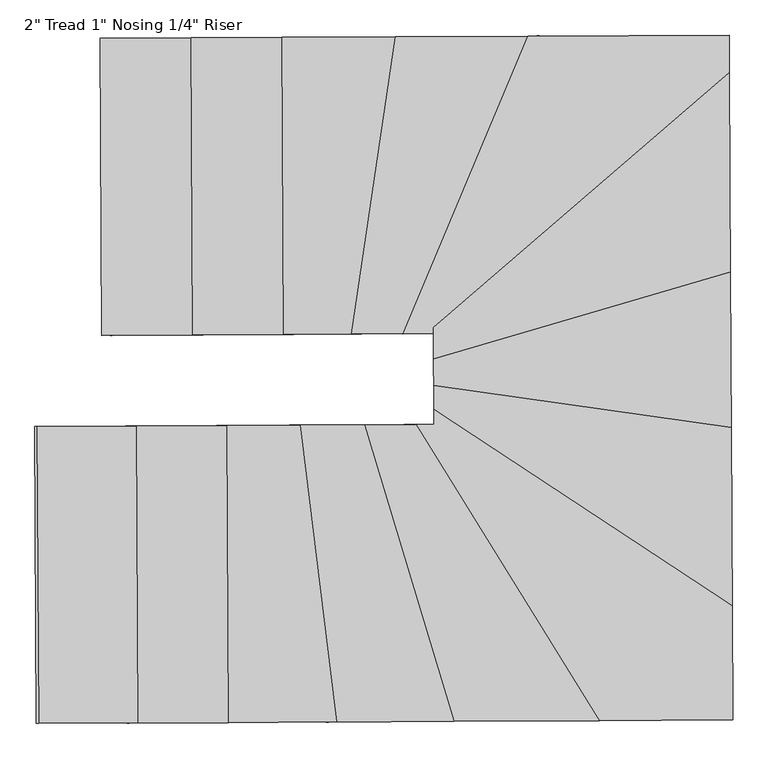
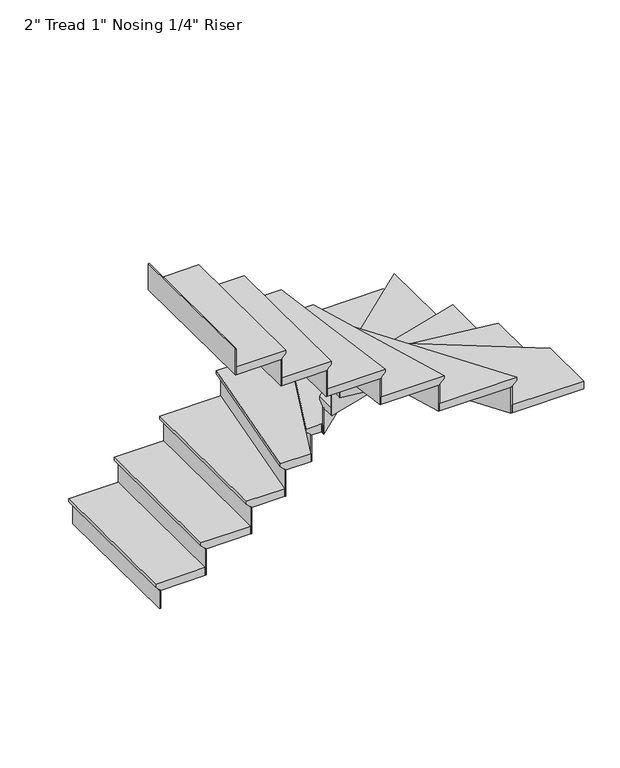
"""IFC4 building model written with IfcOpenShell, lengths in millimetres: stair flight geometry."""

from ifc_helpers import new_model, si_unit, origin, place, context, project, spatial, faceted_brep, source, transform, mapped, element, save


def stair_flight_2f6b2362(model_context):
    return source(origin(), model_context, "Body", "Brep", [
        faceted_brep([(73.5214139, -4197.1296428, 658.2833333), (73.5214139, -4197.1296428, 677.3333333), (68.8012135, -3282.7418259, 677.3333333), (68.8012135, -3282.7418259, 658.2833333), (98.9210755, -4196.9985261, 632.8833333), (94.200875, -3282.6107092, 632.8833333), (378.3173529, -4195.5562427, 677.3333333), (373.5971524, -3281.1684258, 677.3333333), (94.200875, -3282.6107092, 626.5333333), (373.5971524, -3281.1684258, 626.5333333), (378.3173529, -4195.5562427, 626.5333333), (98.9210755, -4196.9985261, 626.5333333)], [[[0, 1, 2, 3]], [[4, 0, 3, 5]], [[2, 1, 6, 7]], [[8, 9, 10, 11]], [[2, 7, 9, 8, 5, 3]], [[8, 11, 4, 5]], [[6, 1, 0, 4, 11, 10]], [[7, 6, 10, 9]]]),
        faceted_brep([(98.9210755, -4196.9985261, 626.5333333), (98.9210755, -4196.9985261, 508.0), (105.2709909, -4196.965747, 508.0), (105.2709909, -4196.965747, 626.5333333), (94.200875, -3282.6107092, 626.5333333), (100.5507904, -3282.5779301, 626.5333333), (100.5507904, -3282.5779301, 508.0), (94.200875, -3282.6107092, 508.0)], [[[0, 1, 2, 3]], [[4, 5, 6, 7]], [[1, 0, 4, 7]], [[2, 1, 7, 6]], [[3, 2, 6, 5]], [[0, 3, 5, 4]]]),
        faceted_brep([(378.3173529, -4195.5562427, 795.8666667), (378.3173529, -4195.5562427, 626.5333333), (384.6672683, -4195.5234635, 626.5333333), (384.6672683, -4195.5234635, 795.8666667), (373.5971524, -3281.1684258, 795.8666667), (379.9470678, -3281.1356466, 795.8666667), (379.9470678, -3281.1356466, 626.5333333), (373.5971524, -3281.1684258, 626.5333333)], [[[0, 1, 2, 3]], [[4, 5, 6, 7]], [[1, 0, 4, 7]], [[2, 1, 7, 6]], [[3, 2, 6, 5]], [[0, 3, 5, 4]]]),
        faceted_brep([(348.1974909, -3281.2995425, 846.6666667), (352.9176913, -4195.6873594, 846.6666667), (657.7136303, -4194.1139592, 846.6666667), (652.9934298, -3279.7261423, 846.6666667), (373.5971524, -3281.1684258, 795.8666667), (652.9934298, -3279.7261423, 795.8666667), (657.7136303, -4194.1139592, 795.8666667), (378.3173529, -4195.5562427, 795.8666667), (373.5971524, -3281.1684258, 802.2166667), (348.1974909, -3281.2995425, 827.6166667), (378.3173529, -4195.5562427, 802.2166667), (352.9176913, -4195.6873594, 827.6166667)], [[[0, 1, 2, 3]], [[4, 5, 6, 7]], [[0, 3, 5, 4, 8, 9]], [[4, 7, 10, 8]], [[2, 1, 11, 10, 7, 6]], [[3, 2, 6, 5]], [[11, 1, 0, 9]], [[10, 11, 9, 8]]]),
        faceted_brep([(657.7136303, -4194.1139592, 965.2), (657.7136303, -4194.1139592, 795.8666667), (664.0635457, -4194.08118, 795.8666667), (664.0635457, -4194.08118, 965.2), (652.9934298, -3279.7261423, 965.2), (659.3433452, -3279.6933631, 965.2), (659.3433452, -3279.6933631, 795.8666667), (652.9934298, -3279.7261423, 795.8666667)], [[[0, 1, 2, 3]], [[4, 5, 6, 7]], [[1, 0, 4, 7]], [[2, 1, 7, 6]], [[3, 2, 6, 5]], [[0, 3, 5, 4]]]),
        faceted_brep([(627.5937682, -3279.857259, 1016.0), (632.3139687, -4194.2450759, 1016.0), (866.9504995, -4193.0338486, 1016.0), (1003.1488336, -3277.9185901, 1016.0), (652.9934298, -3279.7261423, 965.2), (1003.1488336, -3277.9185901, 965.2), (866.9504995, -4193.0338486, 965.2), (657.7136303, -4194.1139592, 965.2), (652.9934298, -3279.7261423, 971.55), (627.5937682, -3279.857259, 996.95), (657.7136303, -4194.1139592, 971.55), (632.3139687, -4194.2450759, 996.95)], [[[0, 1, 2, 3]], [[4, 5, 6, 7]], [[0, 3, 5, 4, 8, 9]], [[4, 7, 10, 8]], [[2, 1, 11, 10, 7, 6]], [[3, 2, 6, 5]], [[11, 1, 0, 9]], [[10, 11, 9, 8]]]),
        faceted_brep([(866.9504995, -4193.0338486, 1134.5333333), (866.9504995, -4193.0338486, 965.2), (873.3753797, -4193.0006825, 965.2), (873.3753797, -4193.0006825, 1134.5333333), (1003.1488336, -3277.9185901, 1134.5333333), (1009.5737138, -3277.885424, 1134.5333333), (1009.5737138, -3277.885424, 965.2), (1003.1488336, -3277.9185901, 965.2)], [[[0, 1, 2, 3]], [[4, 5, 6, 7]], [[1, 0, 4, 7]], [[2, 1, 7, 6]], [[3, 2, 6, 5]], [[0, 3, 5, 4]]]),
        faceted_brep([(977.4493129, -3278.0512547, 1185.3333333), (841.2509788, -4193.1665132, 1185.3333333), (1028.3454494, -4192.2007049, 1185.3333333), (1412.7936505, -3275.8039451, 1185.3333333), (1003.1488336, -3277.9185901, 1134.5333333), (1412.7936505, -3275.8039451, 1134.5333333), (1028.3454494, -4192.2007049, 1134.5333333), (866.9504995, -4193.0338486, 1134.5333333), (1003.1488336, -3277.9185901, 1140.8833333), (977.4493129, -3278.0512547, 1166.2833333), (866.9504995, -4193.0338486, 1140.8833333), (841.2509788, -4193.1665132, 1166.2833333)], [[[0, 1, 2, 3]], [[4, 5, 6, 7]], [[0, 3, 5, 4, 8, 9]], [[4, 7, 10, 8]], [[2, 1, 11, 10, 7, 6]], [[3, 2, 6, 5]], [[11, 1, 0, 9]], [[10, 11, 9, 8]]]),
        faceted_brep([(1028.3454494, -4192.2007049, 1303.8666667), (1028.3454494, -4192.2007049, 1134.5333333), (1035.2465542, -4192.1650804, 1134.5333333), (1035.2465542, -4192.1650804, 1303.8666667), (1412.7936505, -3275.8039451, 1303.8666667), (1419.6947553, -3275.7683206, 1303.8666667), (1419.6947553, -3275.7683206, 1134.5333333), (1412.7936505, -3275.8039451, 1134.5333333)], [[[0, 1, 2, 3]], [[4, 5, 6, 7]], [[1, 0, 4, 7]], [[2, 1, 7, 6]], [[3, 2, 6, 5]], [[0, 3, 5, 4]]]),
        faceted_brep([(2004.5597861, -3422.5660243, 1354.6666667), (2003.7864306, -3272.753156, 1354.6666667), (1385.1892314, -3275.9464431, 1354.6666667), (1000.7410303, -4192.3432028, 1354.6666667), (1094.1188142, -4191.8611734, 1354.6666667), (1094.1970217, -4207.0113762, 1354.6666667), (2003.7864306, -3272.753156, 1303.8666667), (2004.5597861, -3422.5660243, 1303.8666667), (1094.1970217, -4207.0113762, 1303.8666667), (1094.1188142, -4191.8611734, 1303.8666667), (1028.3454494, -4192.2007049, 1303.8666667), (1412.7936505, -3275.8039451, 1303.8666667), (1028.3454494, -4192.2007049, 1310.2166667), (1412.7936505, -3275.8039451, 1310.2166667), (1000.7410303, -4192.3432028, 1335.6166667), (1385.1892314, -3275.9464431, 1335.6166667)], [[[0, 1, 2, 3, 4, 5]], [[6, 7, 8, 9, 10, 11]], [[1, 0, 7, 6]], [[11, 10, 12, 13]], [[4, 3, 14, 12, 10, 9]], [[0, 5, 8, 7]], [[14, 3, 2, 15]], [[12, 14, 15, 13]], [[2, 1, 6, 11, 13, 15]], [[5, 4, 9, 8]]]),
        faceted_brep([(1094.1970217, -4207.0113762, 1473.2), (1094.1970217, -4207.0113762, 1303.8666667), (1094.2401004, -4215.3564963, 1303.8666667), (1094.2401004, -4215.3564963, 1473.2), (2004.5597861, -3422.5660243, 1473.2), (2004.6028648, -3430.9111444, 1473.2), (2004.6028648, -3430.9111444, 1303.8666667), (2004.5597861, -3422.5660243, 1303.8666667)], [[[0, 1, 2, 3]], [[4, 5, 6, 7]], [[1, 0, 4, 7]], [[2, 1, 7, 6]], [[3, 2, 6, 5]], [[0, 3, 5, 4]]]),
        faceted_brep([(2004.3874713, -3389.1855438, 1524.0), (1094.0247069, -4173.6308957, 1524.0), (1094.654759, -4295.6833292, 1524.0), (2007.6910705, -4029.1522065, 1524.0), (2004.5597861, -3422.5660243, 1473.2), (2007.6910705, -4029.1522065, 1473.2), (1094.654759, -4295.6833292, 1473.2), (1094.1970217, -4207.0113762, 1473.2), (2004.5597861, -3422.5660243, 1479.55), (2004.3874713, -3389.1855438, 1504.95), (1094.1970217, -4207.0113762, 1479.55), (1094.0247069, -4173.6308957, 1504.95)], [[[0, 1, 2, 3]], [[4, 5, 6, 7]], [[0, 3, 5, 4, 8, 9]], [[4, 7, 10, 8]], [[3, 2, 6, 5]], [[11, 1, 0, 9]], [[10, 11, 9, 8]], [[2, 1, 11, 10, 7, 6]]]),
        faceted_brep([(1094.654759, -4295.6833292, 1642.5333333), (1094.654759, -4295.6833292, 1473.2), (1094.6888553, -4302.2884051, 1473.2), (1094.6888553, -4302.2884051, 1642.5333333), (2007.6910705, -4029.1522065, 1642.5333333), (2007.7251669, -4035.7572823, 1642.5333333), (2007.7251669, -4035.7572823, 1473.2), (2007.6910705, -4029.1522065, 1473.2)], [[[0, 1, 2, 3]], [[4, 5, 6, 7]], [[1, 0, 4, 7]], [[2, 1, 7, 6]], [[3, 2, 6, 5]], [[0, 3, 5, 4]]]),
        faceted_brep([(2007.5546851, -4002.7319029, 1693.3333333), (1094.5183736, -4269.2630257, 1693.3333333), (1095.0784269, -4377.7554326, 1693.3333333), (2010.1530082, -4506.0738629, 1693.3333333), (2007.6910705, -4029.1522065, 1642.5333333), (2010.1530082, -4506.0738629, 1642.5333333), (1095.0784269, -4377.7554326, 1642.5333333), (1094.654759, -4295.6833292, 1642.5333333), (2007.6910705, -4029.1522065, 1648.8833333), (2007.5546851, -4002.7319029, 1674.2833333), (1094.654759, -4295.6833292, 1648.8833333), (1094.5183736, -4269.2630257, 1674.2833333)], [[[0, 1, 2, 3]], [[4, 5, 6, 7]], [[0, 3, 5, 4, 8, 9]], [[4, 7, 10, 8]], [[2, 1, 11, 10, 7, 6]], [[3, 2, 6, 5]], [[11, 1, 0, 9]], [[10, 11, 9, 8]]]),
        faceted_brep([(1095.0784269, -4377.7554326, 1811.8666667), (1095.0784269, -4377.7554326, 1642.5333333), (1095.1115512, -4384.1722058, 1642.5333333), (1095.1115512, -4384.1722058, 1811.8666667), (2010.1530082, -4506.0738629, 1811.8666667), (2010.1861325, -4512.4906361, 1811.8666667), (2010.1861325, -4512.4906361, 1642.5333333), (2010.1530082, -4506.0738629, 1642.5333333)], [[[0, 1, 2, 3]], [[4, 5, 6, 7]], [[1, 0, 4, 7]], [[2, 1, 7, 6]], [[3, 2, 6, 5]], [[0, 3, 5, 4]]]),
        faceted_brep([(2010.020511, -4480.40677, 1862.6666667), (1094.9459297, -4352.0883397, 1862.6666667), (1095.4823291, -4455.9985745, 1862.6666667), (2013.0146854, -5060.4322638, 1862.6666667), (2010.1530082, -4506.0738629, 1811.8666667), (2013.0146854, -5060.4322638, 1811.8666667), (1095.4823291, -4455.9985745, 1811.8666667), (1095.0784269, -4377.7554326, 1811.8666667), (2010.1530082, -4506.0738629, 1818.2166667), (2010.020511, -4480.40677, 1843.6166667), (1095.0784269, -4377.7554326, 1818.2166667), (1094.9459297, -4352.0883397, 1843.6166667)], [[[0, 1, 2, 3]], [[4, 5, 6, 7]], [[0, 3, 5, 4, 8, 9]], [[4, 7, 10, 8]], [[3, 2, 6, 5]], [[11, 1, 0, 9]], [[10, 11, 9, 8]], [[2, 1, 11, 10, 7, 6]]]),
        faceted_brep([(1095.4823291, -4455.9985745, 1981.2), (1095.4823291, -4455.9985745, 1811.8666667), (1095.5217161, -4463.6285363, 1811.8666667), (1095.5217161, -4463.6285363, 1981.2), (2013.0146854, -5060.4322638, 1981.2), (2013.0540723, -5068.0622255, 1981.2), (2013.0540723, -5068.0622255, 1811.8666667), (2013.0146854, -5060.4322638, 1811.8666667)], [[[0, 1, 2, 3]], [[4, 5, 6, 7]], [[1, 0, 4, 7]], [[2, 1, 7, 6]], [[3, 2, 6, 5]], [[0, 3, 5, 4]]]),
        faceted_brep([(1574.7396622, -5383.1960459, 2032.0), (2014.669115, -5380.9250672, 2032.0), (2012.8571376, -5029.9124167, 2032.0), (1095.3247813, -4425.4787274, 2032.0), (1095.5610976, -4471.2574507, 2032.0), (1010.2079956, -4471.6980556, 2032.0), (2014.669115, -5380.9250672, 1981.2), (1574.7396622, -5383.1960459, 1981.2), (1010.2079956, -4471.6980556, 1981.2), (1095.5610976, -4471.2574507, 1981.2), (1095.4823291, -4455.9985745, 1981.2), (2013.0146854, -5060.4322638, 1981.2), (1095.4823291, -4455.9985745, 1987.55), (2013.0146854, -5060.4322638, 1987.55), (1095.3247813, -4425.4787274, 2012.95), (2012.8571376, -5029.9124167, 2012.95)], [[[0, 1, 2, 3, 4, 5]], [[6, 7, 8, 9, 10, 11]], [[1, 0, 7, 6]], [[11, 10, 12, 13]], [[4, 3, 14, 12, 10, 9]], [[0, 5, 8, 7]], [[14, 3, 2, 15]], [[12, 14, 15, 13]], [[5, 4, 9, 8]], [[2, 1, 6, 11, 13, 15]]]),
        faceted_brep([(1010.2079956, -4471.6980556, 2150.5333333), (1010.2079956, -4471.6980556, 1981.2), (1002.7625472, -4471.7364901, 1981.2), (1002.7625472, -4471.7364901, 2150.5333333), (1574.7396622, -5383.1960459, 2150.5333333), (1567.2942139, -5383.2344803, 2150.5333333), (1567.2942139, -5383.2344803, 1981.2), (1574.7396622, -5383.1960459, 1981.2)], [[[0, 1, 2, 3]], [[4, 5, 6, 7]], [[1, 0, 4, 7]], [[2, 1, 7, 6]], [[3, 2, 6, 5]], [[0, 3, 5, 4]]]),
        faceted_brep([(1604.5214555, -5383.042308, 2201.3333333), (1039.9897889, -4471.5443178, 2201.3333333), (854.9585932, -4472.4994752, 2201.3333333), (1130.3137603, -5385.4902358, 2201.3333333), (1574.7396622, -5383.1960459, 2150.5333333), (1130.3137603, -5385.4902358, 2150.5333333), (854.9585932, -4472.4994752, 2150.5333333), (1010.2079956, -4471.6980556, 2150.5333333), (1574.7396622, -5383.1960459, 2156.8833333), (1604.5214555, -5383.042308, 2182.2833333), (1010.2079956, -4471.6980556, 2156.8833333), (1039.9897889, -4471.5443178, 2182.2833333)], [[[0, 1, 2, 3]], [[4, 5, 6, 7]], [[0, 3, 5, 4, 8, 9]], [[4, 7, 10, 8]], [[2, 1, 11, 10, 7, 6]], [[3, 2, 6, 5]], [[11, 1, 0, 9]], [[10, 11, 9, 8]]]),
        faceted_brep([(854.9585932, -4472.4994752, 2319.8666667), (854.9585932, -4472.4994752, 2150.5333333), (848.3363877, -4472.53366, 2150.5333333), (848.3363877, -4472.53366, 2319.8666667), (1130.3137603, -5385.4902358, 2319.8666667), (1123.6915548, -5385.5244206, 2319.8666667), (1123.6915548, -5385.5244206, 2150.5333333), (1130.3137603, -5385.4902358, 2150.5333333)], [[[0, 1, 2, 3]], [[4, 5, 6, 7]], [[1, 0, 4, 7]], [[2, 1, 7, 6]], [[3, 2, 6, 5]], [[0, 3, 5, 4]]]),
        faceted_brep([(1156.8025822, -5385.3534967, 2370.6666667), (881.4474152, -4472.3627361, 2370.6666667), (657.851655, -4473.5169694, 2370.6666667), (770.454123, -5387.3478826, 2370.6666667), (1130.3137603, -5385.4902358, 2319.8666667), (770.454123, -5387.3478826, 2319.8666667), (657.851655, -4473.5169694, 2319.8666667), (854.9585932, -4472.4994752, 2319.8666667), (1130.3137603, -5385.4902358, 2326.2166667), (1156.8025822, -5385.3534967, 2351.6166667), (854.9585932, -4472.4994752, 2326.2166667), (881.4474152, -4472.3627361, 2351.6166667)], [[[0, 1, 2, 3]], [[4, 5, 6, 7]], [[0, 3, 5, 4, 8, 9]], [[4, 7, 10, 8]], [[2, 1, 11, 10, 7, 6]], [[3, 2, 6, 5]], [[11, 1, 0, 9]], [[10, 11, 9, 8]]]),
        faceted_brep([(657.851655, -4473.5169694, 2489.2), (657.851655, -4473.5169694, 2319.8666667), (651.457697, -4473.5499759, 2319.8666667), (651.457697, -4473.5499759, 2489.2), (770.454123, -5387.3478826, 2489.2), (764.060165, -5387.3808891, 2489.2), (764.060165, -5387.3808891, 2319.8666667), (770.454123, -5387.3478826, 2319.8666667)], [[[0, 1, 2, 3]], [[4, 5, 6, 7]], [[1, 0, 4, 7]], [[2, 1, 7, 6]], [[3, 2, 6, 5]], [[0, 3, 5, 4]]]),
        faceted_brep([(796.0299553, -5387.2158565, 2540.0), (683.4274873, -4473.3849433, 2540.0), (432.5726821, -4474.6798916, 2540.0), (437.2928826, -5389.0677085, 2540.0), (770.454123, -5387.3478826, 2489.2), (437.2928826, -5389.0677085, 2489.2), (432.5726821, -4474.6798916, 2489.2), (657.851655, -4473.5169694, 2489.2), (770.454123, -5387.3478826, 2495.55), (796.0299553, -5387.2158565, 2520.95), (657.851655, -4473.5169694, 2495.55), (683.4274873, -4473.3849433, 2520.95)], [[[0, 1, 2, 3]], [[4, 5, 6, 7]], [[0, 3, 5, 4, 8, 9]], [[4, 7, 10, 8]], [[2, 1, 11, 10, 7, 6]], [[3, 2, 6, 5]], [[11, 1, 0, 9]], [[10, 11, 9, 8]]]),
        faceted_brep([(432.5726821, -4474.6798916, 2658.5333333), (432.5726821, -4474.6798916, 2489.2), (426.2227667, -4474.7126708, 2489.2), (426.2227667, -4474.7126708, 2658.5333333), (437.2928826, -5389.0677085, 2658.5333333), (430.9429672, -5389.1004877, 2658.5333333), (430.9429672, -5389.1004877, 2489.2), (437.2928826, -5389.0677085, 2489.2)], [[[0, 1, 2, 3]], [[4, 5, 6, 7]], [[1, 0, 4, 7]], [[2, 1, 7, 6]], [[3, 2, 6, 5]], [[0, 3, 5, 4]]]),
        faceted_brep([(462.6925441, -5388.9365918, 2709.3333333), (457.9723437, -4474.5487749, 2709.3333333), (153.1764047, -4476.1221751, 2709.3333333), (157.8966052, -5390.509992, 2709.3333333), (437.2928826, -5389.0677085, 2658.5333333), (157.8966052, -5390.509992, 2658.5333333), (153.1764047, -4476.1221751, 2658.5333333), (432.5726821, -4474.6798916, 2658.5333333), (437.2928826, -5389.0677085, 2664.8833333), (462.6925441, -5388.9365918, 2690.2833333), (432.5726821, -4474.6798916, 2664.8833333), (457.9723437, -4474.5487749, 2690.2833333)], [[[0, 1, 2, 3]], [[4, 5, 6, 7]], [[0, 3, 5, 4, 8, 9]], [[4, 7, 10, 8]], [[2, 1, 11, 10, 7, 6]], [[3, 2, 6, 5]], [[11, 1, 0, 9]], [[10, 11, 9, 8]]]),
        faceted_brep([(153.1764047, -4476.1221751, 2827.8666667), (153.1764047, -4476.1221751, 2658.5333333), (146.8264893, -4476.1549542, 2658.5333333), (146.8264893, -4476.1549542, 2827.8666667), (157.8966052, -5390.509992, 2827.8666667), (151.5466898, -5390.5427711, 2827.8666667), (151.5466898, -5390.5427711, 2658.5333333), (157.8966052, -5390.509992, 2658.5333333)], [[[0, 1, 2, 3]], [[4, 5, 6, 7]], [[1, 0, 4, 7]], [[2, 1, 7, 6]], [[3, 2, 6, 5]], [[0, 3, 5, 4]]]),
        faceted_brep([(-126.2198726, -4477.5644585, 2997.2), (-126.2198726, -4477.5644585, 2827.8666667), (-132.569788, -4477.5972377, 2827.8666667), (-132.569788, -4477.5972377, 2997.2), (-121.4996722, -5391.9522754, 2997.2), (-127.8495876, -5391.9850546, 2997.2), (-127.8495876, -5391.9850546, 2827.8666667), (-121.4996722, -5391.9522754, 2827.8666667)], [[[0, 1, 2, 3]], [[4, 5, 6, 7]], [[1, 0, 4, 7]], [[2, 1, 7, 6]], [[3, 2, 6, 5]], [[0, 3, 5, 4]]]),
        faceted_brep([(183.2962668, -5390.3788753, 2878.6666667), (178.5760663, -4475.9910584, 2878.6666667), (-126.2198726, -4477.5644585, 2878.6666667), (-121.4996722, -5391.9522754, 2878.6666667), (157.8966052, -5390.509992, 2827.8666667), (-121.4996722, -5391.9522754, 2827.8666667), (-126.2198726, -4477.5644585, 2827.8666667), (153.1764047, -4476.1221751, 2827.8666667), (157.8966052, -5390.509992, 2834.2166667), (183.2962668, -5390.3788753, 2859.6166667), (153.1764047, -4476.1221751, 2834.2166667), (178.5760663, -4475.9910584, 2859.6166667)], [[[0, 1, 2, 3]], [[4, 5, 6, 7]], [[0, 3, 5, 4, 8, 9]], [[4, 7, 10, 8]], [[2, 1, 11, 10, 7, 6]], [[3, 2, 6, 5]], [[11, 1, 0, 9]], [[10, 11, 9, 8]]]),
    ])


if __name__ == "__main__":
    model = new_model("IFC4")
    model_context = context("Model", 3, world=origin())
    ifc_project = project(units=[si_unit("LENGTHUNIT", "METRE", prefix="MILLI")], contexts=[model_context])
    site = spatial("IfcSite", under=ifc_project)
    building = spatial("IfcBuilding", under=site)
    placement = place(None, origin())
    stair_flight_shape = stair_flight_2f6b2362(model_context)
    element("IfcStairFlight", 1, ObjectType="2\" Tread 1\" Nosing 1/4\" Riser", at=placement, inside=building, context=model_context, shape_type="MappedRepresentation", body=[
        mapped(stair_flight_shape, transform((0.0, 0.0, 0.0), x_axis=(1.0, 0.0, 0.0), y_axis=(0.0, 1.0, 0.0), z_axis=(0.0, 0.0, 1.0))),
    ])
    save(model, "model.ifc")
